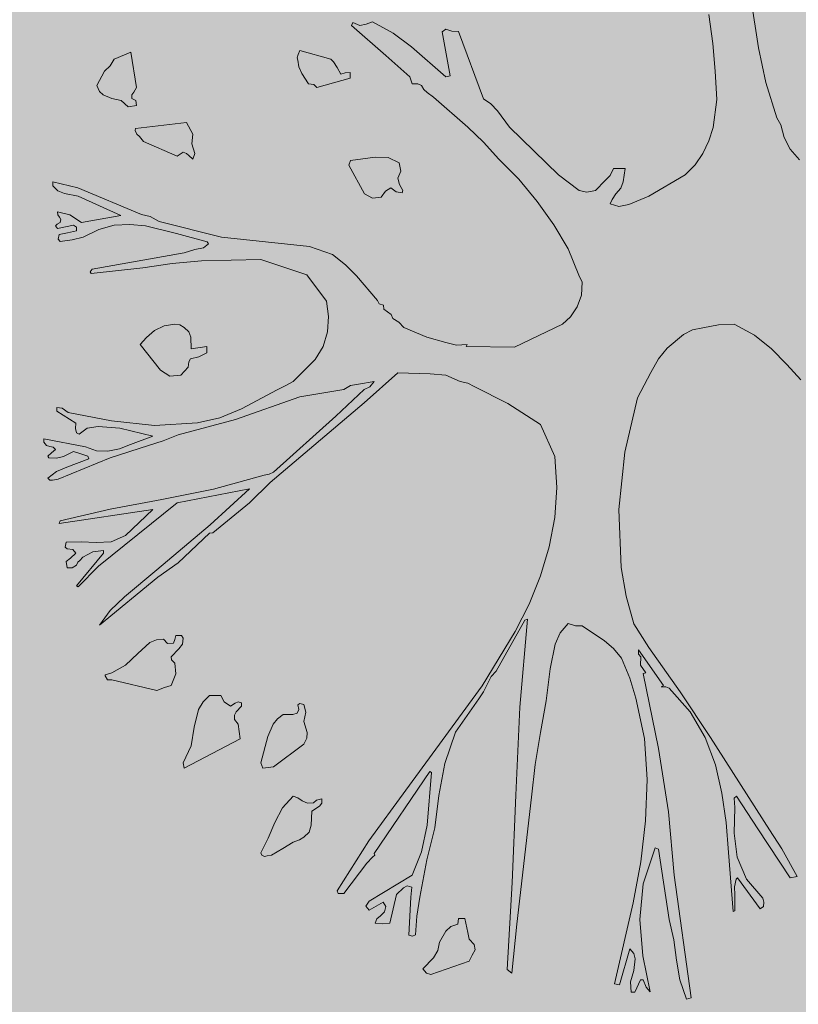
# Model space of a CAD drawing. Units: inches. Extents: x 84 to 1044, y -280 to 906.
# Tile 83 of 105: x 831.19 to 844.48, y 408.65 to 425.45. Entities that reach past the tile are written whole.
import ezdxf

# ---------------------------------------------------------------- set-up
doc = ezdxf.new("R2010")
doc.units = ezdxf.units.IN
doc.layers.add('A-ANNO-DIMS', color=2, linetype='Continuous', lineweight=18)
doc.layers.add('L-PLNT', color=114, linetype='Continuous', lineweight=15)
doc.layers.add('L-PLNT-PATT', color=9, linetype='Continuous', lineweight=9, true_color=0xafd9aa)
doc.styles.get("Standard").update_dxf_attribs({"font": 'arial.ttf'})
doc.dimstyles.get("Standard").update_dxf_attribs({"dimtxt": 0.18, "dimasz": 0.18, "dimexe": 0.18, "dimexo": 0.0625, "dimgap": 0.09, "dimtad": 0, "dimtih": 1, "dimtoh": 1, "dimdec": 4, "dimzin": 0, "dimdsep": 46, "dimtxsty": 'Standard', "dimcen": 0.09, "dimadec": 0, "dimazin": 0, "dimtfac": 1, "dimtdec": 4, "dimtofl": 0, "dimtmove": 0, "dimatfit": 3, "dimfxl": 1, "dimtolj": 1, "dimtzin": 0, "dimarcsym": 0})

# ---------------------------------------------------------------- blocks, each defined once
blk = doc.blocks.new('A$C37E508DF')
for p, q in [((0.7911, 1.1436), (0.8027, 1.0677)), ((0.7512, 1.0728), (0.7469, 1.1054)), ((0.3456, 1.093), (0.3469, 1.0964)), ((0.3469, 1.0964), (0.355, 1.093)), ((0.355, 1.093), (0.3619, 1.0943)), ((0.3619, 1.0943), (0.3692, 1.0968)), ((0.3692, 1.0968), (0.3923, 1.0844)), ((0.3842, 1.0591), (0.3456, 1.093)), ((0.3923, 1.0844), (0.4129, 1.069)), ((0.4472, 1.0857), (0.4515, 1.0887)), ((0.4562, 1.0364), (0.4472, 1.0857)), ((0.4515, 1.0887), (0.4584, 1.0865)), ((0.4584, 1.0865), (0.4657, 1.0861)), ((0.4657, 1.0861), (0.4939, 1.0107)), ((0.7538, 1.0415), (0.7512, 1.0728)), ((0.0789, 1.0552), (0.0978, 1.063)), ((0.0978, 1.063), (0.1042, 1.0231)), ((0.2856, 1.0604), (0.2877, 1.0647)), ((0.2877, 1.0647), (0.3224, 1.0552)), ((0.4129, 1.069), (0.4515, 1.0351)), ((0.8027, 1.0677), (0.8108, 1.0287)), ((0.0746, 1.0475), (0.0789, 1.0552)), ((0.2847, 1.0565), (0.2856, 1.0604)), ((0.2851, 1.054), (0.2847, 1.0565)), ((0.2864, 1.0463), (0.2851, 1.054)), ((0.3224, 1.0552), (0.3255, 1.0522)), ((0.3255, 1.0522), (0.3293, 1.0458)), ((0.4112, 1.0351), (0.3842, 1.0591)), ((0.0596, 1.0257), (0.0682, 1.0415)), ((0.0682, 1.0415), (0.0746, 1.0475)), ((0.2899, 1.039), (0.2864, 1.0463)), ((0.3293, 1.0458), (0.3336, 1.0381)), ((0.3336, 1.0381), (0.3383, 1.0398)), ((0.3383, 1.0398), (0.3439, 1.0402)), ((0.3439, 1.0402), (0.3439, 1.0338)), ((0.7559, 1.0098), (0.7538, 1.0415)), ((0.2972, 1.0274), (0.2899, 1.039)), ((0.3439, 1.0338), (0.3066, 1.0231)), ((0.4138, 1.0274), (0.4112, 1.0351)), ((0.4515, 1.0351), (0.4562, 1.0364)), ((0.8108, 1.0287), (0.8233, 0.9892)), ((0.0626, 1.0188), (0.0596, 1.0257)), ((0.0665, 1.0149), (0.0626, 1.0188)), ((0.1012, 1.018), (0.099, 1.0149)), ((0.1042, 1.0231), (0.1012, 1.018)), ((0.3032, 1.0265), (0.2972, 1.0274)), ((0.3066, 1.0231), (0.3032, 1.0265)), ((0.4202, 1.0274), (0.4138, 1.0274)), ((0.4241, 1.0257), (0.4202, 1.0274)), ((0.4267, 1.0209), (0.4241, 1.0257)), ((0.4305, 1.0175), (0.4267, 1.0209)), ((0.4378, 1.0124), (0.4305, 1.0175)), ((0.0763, 1.0111), (0.0665, 1.0149)), ((0.087, 1.0085), (0.0763, 1.0111)), ((0.0948, 1.0016), (0.087, 1.0085)), ((0.099, 1.0149), (0.099, 1.0111)), ((0.099, 1.0111), (0.1033, 1.0085)), ((0.1033, 1.0085), (0.1042, 1.0029)), ((0.476, 0.9789), (0.4378, 1.0124)), ((0.4939, 1.0107), (0.5021, 1.0051)), ((0.7516, 0.9785), (0.7559, 1.0098)), ((0.1042, 1.0029), (0.0948, 1.0016)), ((0.5021, 1.0051), (0.5094, 0.9969)), ((0.5094, 0.9969), (0.5231, 0.9789)), ((0.1029, 0.9772), (0.1604, 0.9841)), ((0.1604, 0.9841), (0.1672, 0.9708)), ((0.8233, 0.9892), (0.8275, 0.9815)), ((0.1025, 0.9751), (0.1029, 0.9772)), ((0.1046, 0.9708), (0.1025, 0.9751)), ((0.4939, 0.9618), (0.476, 0.9789)), ((0.5231, 0.9789), (0.578, 0.9253)), ((0.7469, 0.9635), (0.7516, 0.9785)), ((0.8275, 0.9815), (0.8314, 0.9673)), ((0.1076, 0.9682), (0.1046, 0.9708)), ((0.1119, 0.9626), (0.1076, 0.9682)), ((0.1496, 0.9463), (0.1119, 0.9626)), ((0.1672, 0.9708), (0.1664, 0.9601)), ((0.5111, 0.9429), (0.4939, 0.9618)), ((0.7401, 0.9493), (0.7469, 0.9635)), ((0.8314, 0.9673), (0.8383, 0.954)), ((0.1565, 0.9506), (0.1496, 0.9463)), ((0.1604, 0.9493), (0.1565, 0.9506)), ((0.1664, 0.9601), (0.1698, 0.9493)), ((0.8383, 0.954), (0.8486, 0.942)), ((0.1629, 0.9468), (0.1604, 0.9493)), ((0.1672, 0.9429), (0.1629, 0.9468)), ((0.1698, 0.9493), (0.1672, 0.9429)), ((0.3426, 0.936), (0.3443, 0.9412)), ((0.3443, 0.9412), (0.3722, 0.9451)), ((0.3722, 0.9451), (0.3868, 0.9446)), ((0.3868, 0.9446), (0.3992, 0.9386)), ((0.5334, 0.9202), (0.5111, 0.9429)), ((0.7315, 0.9365), (0.7401, 0.9493)), ((0.3602, 0.9039), (0.3426, 0.936)), ((0.4009, 0.9292), (0.3975, 0.9215)), ((0.3992, 0.9386), (0.4009, 0.9292)), ((0.6359, 0.9245), (0.6397, 0.9322)), ((0.6397, 0.9322), (0.653, 0.9322)), ((0.653, 0.9322), (0.6505, 0.9172)), ((0.7203, 0.9253), (0.7315, 0.9365)), ((0.3975, 0.9215), (0.3996, 0.9142)), ((0.554, 0.8953), (0.5334, 0.9202)), ((0.578, 0.9253), (0.6011, 0.9077)), ((0.6196, 0.9077), (0.6303, 0.9189)), ((0.6303, 0.9189), (0.6359, 0.9245)), ((0.6796, 0.9013), (0.7203, 0.9253)), ((0.0103, 0.9129), (0.0103, 0.9172)), ((0.0103, 0.9172), (0.0382, 0.9107)), ((0.0159, 0.9073), (0.0103, 0.9129)), ((0.0232, 0.9043), (0.0159, 0.9073)), ((0.0382, 0.9107), (0.1098, 0.8807)), ((0.3838, 0.9069), (0.379, 0.9)), ((0.3898, 0.9107), (0.3838, 0.9069)), ((0.3958, 0.906), (0.3898, 0.9107)), ((0.3996, 0.9142), (0.4031, 0.9077)), ((0.4031, 0.9077), (0.4026, 0.9052)), ((0.6011, 0.9077), (0.6097, 0.9056)), ((0.6097, 0.9056), (0.6196, 0.9077)), ((0.6479, 0.9103), (0.6423, 0.9039)), ((0.6505, 0.9172), (0.6479, 0.9103)), ((0.0386, 0.9013), (0.0232, 0.9043)), ((0.0866, 0.8794), (0.0386, 0.9013)), ((0.3692, 0.8992), (0.3602, 0.9039)), ((0.379, 0.9), (0.3692, 0.8992)), ((0.4026, 0.9052), (0.3958, 0.906)), ((0.5728, 0.8691), (0.554, 0.8953)), ((0.6384, 0.8974), (0.6359, 0.8927)), ((0.6423, 0.9039), (0.6384, 0.8974)), ((0.6569, 0.8919), (0.6796, 0.9013)), ((0.6359, 0.8927), (0.6457, 0.8897)), ((0.6457, 0.8897), (0.6569, 0.8919)), ((0.0159, 0.8803), (0.0154, 0.8837)), ((0.0154, 0.8837), (0.0292, 0.8803)), ((0.0176, 0.8777), (0.0159, 0.8803)), ((0.0193, 0.8752), (0.0176, 0.8777)), ((0.0184, 0.8717), (0.0193, 0.8752)), ((0.0292, 0.8803), (0.0424, 0.8717)), ((0.0424, 0.8717), (0.0866, 0.8794)), ((0.1098, 0.8807), (0.1196, 0.8786)), ((0.1196, 0.8786), (0.1295, 0.873)), ((0.0133, 0.8679), (0.015, 0.87)), ((0.0154, 0.8649), (0.0133, 0.8679)), ((0.015, 0.87), (0.0184, 0.8717)), ((0.0334, 0.8687), (0.0154, 0.8649)), ((0.0266, 0.8602), (0.0369, 0.8623)), ((0.0369, 0.8666), (0.0334, 0.8687)), ((0.0369, 0.8623), (0.0369, 0.8666)), ((0.0617, 0.864), (0.0442, 0.8554)), ((0.0789, 0.8687), (0.0617, 0.864)), ((0.0965, 0.8696), (0.0789, 0.8687)), ((0.1141, 0.8679), (0.0965, 0.8696)), ((0.1492, 0.8593), (0.1141, 0.8679)), ((0.1295, 0.873), (0.1994, 0.8554)), ((0.5887, 0.8421), (0.5728, 0.8691)), ((0.0163, 0.8529), (0.0171, 0.8584)), ((0.0184, 0.8503), (0.0163, 0.8529)), ((0.0171, 0.8584), (0.0266, 0.8602)), ((0.0317, 0.8524), (0.0184, 0.8503)), ((0.0442, 0.8554), (0.0317, 0.8524)), ((0.1835, 0.8499), (0.1492, 0.8593)), ((0.1994, 0.8554), (0.2984, 0.8447)), ((0.1578, 0.8378), (0.1698, 0.8413)), ((0.1698, 0.8413), (0.1792, 0.8434)), ((0.1792, 0.8434), (0.1848, 0.8477)), ((0.1848, 0.8477), (0.1835, 0.8499)), ((0.2984, 0.8447), (0.3242, 0.8357)), ((0.6007, 0.8125), (0.5887, 0.8421)), ((0.0545, 0.8194), (0.1578, 0.8378)), ((0.2436, 0.8301), (0.1771, 0.8288)), ((0.2954, 0.813), (0.2436, 0.8301)), ((0.3242, 0.8357), (0.3387, 0.8241)), ((0.0519, 0.8164), (0.0545, 0.8194)), ((0.1111, 0.8207), (0.0532, 0.8143)), ((0.1441, 0.8258), (0.1111, 0.8207)), ((0.1771, 0.8288), (0.1441, 0.8258)), ((0.3387, 0.8241), (0.3512, 0.8117)), ((0.0532, 0.8143), (0.0519, 0.8164)), ((0.3173, 0.7834), (0.2954, 0.813)), ((0.3512, 0.8117), (0.3748, 0.7842)), ((0.6046, 0.8048), (0.6007, 0.8125)), ((0.6037, 0.7903), (0.6046, 0.8048)), ((0.599, 0.777), (0.6037, 0.7903)), ((0.3199, 0.7662), (0.3173, 0.7834)), ((0.3748, 0.7842), (0.3765, 0.7804)), ((0.3765, 0.7804), (0.3816, 0.7791)), ((0.3816, 0.7791), (0.382, 0.7744)), ((0.382, 0.7744), (0.3859, 0.7714)), ((0.5913, 0.7658), (0.599, 0.777)), ((0.3186, 0.7491), (0.3199, 0.7662)), ((0.3859, 0.7714), (0.3902, 0.7684)), ((0.3902, 0.7684), (0.3919, 0.7641)), ((0.3919, 0.7641), (0.3988, 0.7598)), ((0.5823, 0.7577), (0.5913, 0.7658)), ((0.1244, 0.7504), (0.1351, 0.7559)), ((0.1351, 0.7559), (0.1471, 0.7577)), ((0.1471, 0.7577), (0.1527, 0.7568)), ((0.1527, 0.7568), (0.1578, 0.7538)), ((0.1578, 0.7538), (0.1629, 0.7491)), ((0.3988, 0.7598), (0.4043, 0.7538)), ((0.4043, 0.7538), (0.4301, 0.7431)), ((0.5287, 0.7319), (0.5823, 0.7577)), ((0.7401, 0.7534), (0.7285, 0.7512)), ((0.7577, 0.7568), (0.7401, 0.7534)), ((0.7752, 0.7577), (0.7577, 0.7568)), ((0.798, 0.7452), (0.7752, 0.7577)), ((0.1081, 0.7349), (0.1153, 0.7427)), ((0.1153, 0.7427), (0.1244, 0.7504)), ((0.1629, 0.7491), (0.1651, 0.7431)), ((0.1651, 0.7431), (0.1655, 0.7298)), ((0.3139, 0.7324), (0.3186, 0.7491)), ((0.4301, 0.7431), (0.4515, 0.7371)), ((0.7182, 0.7461), (0.7002, 0.7307)), ((0.7285, 0.7512), (0.7182, 0.7461)), ((0.8173, 0.7298), (0.798, 0.7452)), ((0.1312, 0.7058), (0.1081, 0.7349)), ((0.1655, 0.7298), (0.1831, 0.7324)), ((0.1831, 0.7324), (0.1831, 0.7255)), ((0.3049, 0.7178), (0.3139, 0.7324)), ((0.4515, 0.7371), (0.4635, 0.7341)), ((0.4635, 0.7341), (0.4755, 0.7349)), ((0.4755, 0.7349), (0.4742, 0.7324)), ((0.4742, 0.7324), (0.5287, 0.7319)), ((0.7002, 0.7307), (0.6903, 0.7186)), ((0.8344, 0.7122), (0.8173, 0.7298)), ((0.1646, 0.7186), (0.1629, 0.7152)), ((0.1741, 0.7208), (0.1646, 0.7186)), ((0.1831, 0.7255), (0.1741, 0.7208)), ((0.6903, 0.7186), (0.6818, 0.7032)), ((0.1621, 0.7092), (0.1539, 0.7002)), ((0.1629, 0.7152), (0.1621, 0.7092)), ((0.28, 0.6933), (0.3049, 0.7178)), ((0.8503, 0.6951), (0.8344, 0.7122)), ((0.1415, 0.6994), (0.1312, 0.7058)), ((0.1539, 0.7002), (0.1415, 0.6994)), ((0.3975, 0.7028), (0.3598, 0.6693)), ((0.4339, 0.7019), (0.3975, 0.7028)), ((0.4515, 0.7002), (0.4339, 0.7019)), ((0.4674, 0.6933), (0.4515, 0.7002)), ((0.6818, 0.7032), (0.6667, 0.6749)), ((0.262, 0.6839), (0.271, 0.6882)), ((0.271, 0.6882), (0.28, 0.6933)), ((0.3443, 0.6886), (0.337, 0.6843)), ((0.3533, 0.6903), (0.3443, 0.6886)), ((0.3709, 0.6933), (0.3533, 0.6903)), ((0.3598, 0.6843), (0.3662, 0.6873)), ((0.3662, 0.6873), (0.3709, 0.6933)), ((0.476, 0.6912), (0.4674, 0.6933)), ((0.4832, 0.6878), (0.476, 0.6912)), ((0.521, 0.6685), (0.4832, 0.6878)), ((0.2877, 0.6762), (0.2152, 0.6505)), ((0.2221, 0.6625), (0.262, 0.6839)), ((0.337, 0.6843), (0.2877, 0.6762)), ((0.328, 0.6543), (0.3598, 0.6843)), ((0.6667, 0.6749), (0.6526, 0.614)), ((0.0146, 0.6599), (0.0146, 0.6642)), ((0.0146, 0.6642), (0.0206, 0.6633)), ((0.0206, 0.6633), (0.0274, 0.6586)), ((0.3598, 0.6693), (0.2543, 0.5797)), ((0.5578, 0.6449), (0.521, 0.6685)), ((0.036, 0.6466), (0.0146, 0.6599)), ((0.0274, 0.6586), (0.0759, 0.6492)), ((0.1728, 0.647), (0.1977, 0.6526)), ((0.1977, 0.6526), (0.2221, 0.6625)), ((0.2581, 0.5913), (0.328, 0.6543)), ((0.0356, 0.6406), (0.036, 0.6466)), ((0.0609, 0.6428), (0.0489, 0.641)), ((0.0853, 0.641), (0.0609, 0.6428)), ((0.0759, 0.6492), (0.1244, 0.644)), ((0.1244, 0.644), (0.1728, 0.647)), ((0.2152, 0.6505), (0.1509, 0.6333)), ((0.5737, 0.6089), (0.5578, 0.6449)), ((0.0369, 0.6355), (0.0356, 0.6406)), ((0.0399, 0.6342), (0.0369, 0.6355)), ((0.0489, 0.641), (0.0399, 0.6342)), ((0.1226, 0.632), (0.0853, 0.641)), ((0.0973, 0.6226), (0.1226, 0.632)), ((0.1509, 0.6333), (0.1342, 0.6265)), ((0, 0.629), (0.0467, 0.62)), ((0, 0.6252), (0, 0.629)), ((0.003, 0.6213), (0, 0.6252)), ((0.0069, 0.6204), (0.003, 0.6213)), ((0.0107, 0.6196), (0.0069, 0.6204)), ((0.0133, 0.617), (0.0107, 0.6196)), ((0.0467, 0.62), (0.0592, 0.6153)), ((0.1175, 0.6213), (0.0746, 0.6076)), ((0.0849, 0.6175), (0.0973, 0.6226)), ((0.1342, 0.6265), (0.1175, 0.6213)), ((0.0047, 0.6093), (0.0086, 0.6132)), ((0.0056, 0.6076), (0.0047, 0.6093)), ((0.0086, 0.6132), (0.0133, 0.617)), ((0.0223, 0.6089), (0.0141, 0.6072)), ((0.0334, 0.6145), (0.0223, 0.6089)), ((0.0416, 0.6119), (0.0334, 0.6145)), ((0.0493, 0.6093), (0.0416, 0.6119)), ((0.0506, 0.6063), (0.0493, 0.6093)), ((0.0592, 0.6153), (0.072, 0.6149)), ((0.072, 0.6149), (0.0849, 0.6175)), ((0.5763, 0.5741), (0.5737, 0.6089)), ((0.6526, 0.614), (0.6457, 0.5497)), ((0.0141, 0.6072), (0.0056, 0.6076)), ((0.0141, 0.5921), (0.0257, 0.5969)), ((0.0746, 0.6076), (0.0163, 0.5836)), ((0.0257, 0.5969), (0.0506, 0.6063)), ((0.0047, 0.5849), (0.0141, 0.5921)), ((0.1904, 0.5724), (0.2474, 0.5879)), ((0.2474, 0.5879), (0.253, 0.5892)), ((0.253, 0.5892), (0.2581, 0.5913)), ((0.0069, 0.5823), (0.0047, 0.5849)), ((0.0099, 0.5823), (0.0069, 0.5823)), ((0.0163, 0.5836), (0.0099, 0.5823)), ((0.2543, 0.5797), (0.2311, 0.557)), ((0.1325, 0.5608), (0.1904, 0.5724)), ((0.2311, 0.5729), (0.1496, 0.557)), ((0.1869, 0.5325), (0.2311, 0.5729)), ((0.5737, 0.5407), (0.5763, 0.5741)), ((0.1496, 0.557), (0.0613, 0.4858)), ((0.0746, 0.5501), (0.1325, 0.5608)), ((0.2311, 0.557), (0.1899, 0.5235)), ((0.1226, 0.5497), (0.0171, 0.5338)), ((0.0184, 0.5368), (0.0746, 0.5501)), ((0.0917, 0.5205), (0.1226, 0.5497)), ((0.6457, 0.5497), (0.6483, 0.4845)), ((0.0171, 0.5338), (0.0184, 0.5368)), ((0.1269, 0.482), (0.1869, 0.5325)), ((0.5677, 0.5077), (0.5737, 0.5407)), ((0.0755, 0.5133), (0.0917, 0.5205)), ((0.1861, 0.5231), (0.1509, 0.4897)), ((0.1899, 0.5235), (0.1861, 0.5231)), ((0.024, 0.5072), (0.0253, 0.5128)), ((0.0253, 0.5128), (0.042, 0.5133)), ((0.042, 0.5133), (0.0587, 0.5124)), ((0.0587, 0.5124), (0.0755, 0.5133)), ((0.0262, 0.5055), (0.024, 0.5072)), ((0.0326, 0.5047), (0.0262, 0.5055)), ((0.03, 0.4948), (0.036, 0.5004)), ((0.036, 0.5004), (0.0326, 0.5047)), ((0.0369, 0.4639), (0.0669, 0.5004)), ((0.0549, 0.5021), (0.0437, 0.4961)), ((0.0669, 0.5034), (0.0549, 0.5021)), ((0.0669, 0.5004), (0.0669, 0.5034)), ((0.5578, 0.4751), (0.5677, 0.5077)), ((0.0253, 0.491), (0.03, 0.4948)), ((0.0262, 0.4841), (0.0253, 0.491)), ((0.0369, 0.4871), (0.0317, 0.4841)), ((0.0382, 0.4905), (0.0369, 0.4871)), ((0.0403, 0.4922), (0.0382, 0.4905)), ((0.0437, 0.4961), (0.0403, 0.4922)), ((0.1509, 0.4897), (0.1282, 0.4734)), ((0.0317, 0.4841), (0.0262, 0.4841)), ((0.0613, 0.4858), (0.0386, 0.4627)), ((0.0905, 0.4515), (0.1269, 0.482)), ((0.6483, 0.4845), (0.6539, 0.4524)), ((0.1282, 0.4734), (0.0626, 0.4198)), ((0.545, 0.4434), (0.5578, 0.4751)), ((0.0386, 0.4627), (0.0369, 0.4639)), ((0.0746, 0.4361), (0.0905, 0.4515)), ((0.5295, 0.4125), (0.545, 0.4434)), ((0.6539, 0.4524), (0.6625, 0.4211)), ((0.0626, 0.4198), (0.0746, 0.4361)), ((0.5403, 0.4254), (0.5081, 0.3679)), ((0.5347, 0.3276), (0.5433, 0.4266)), ((0.5433, 0.4266), (0.5403, 0.4254)), ((0.5887, 0.4215), (0.5797, 0.4112)), ((0.5969, 0.4189), (0.5887, 0.4215)), ((0.6625, 0.4211), (0.6796, 0.3945)), ((0.4922, 0.3516), (0.5295, 0.4125)), ((0.5797, 0.4112), (0.5741, 0.3983)), ((0.6046, 0.4189), (0.5969, 0.4189)), ((0.6295, 0.4022), (0.6046, 0.4189)), ((0.1055, 0.388), (0.1192, 0.4001)), ((0.1192, 0.4001), (0.1265, 0.4031)), ((0.1265, 0.4031), (0.1346, 0.4039)), ((0.1346, 0.4039), (0.1389, 0.3992)), ((0.1389, 0.3992), (0.1458, 0.3996)), ((0.1458, 0.3996), (0.1471, 0.4035)), ((0.1471, 0.4035), (0.1484, 0.4082)), ((0.1484, 0.4082), (0.1548, 0.4082)), ((0.1556, 0.3983), (0.1518, 0.3932)), ((0.1548, 0.4082), (0.1565, 0.4052)), ((0.1565, 0.4052), (0.1556, 0.3983)), ((0.5741, 0.3983), (0.5686, 0.3705)), ((0.6397, 0.3936), (0.6295, 0.4022)), ((0.0917, 0.3748), (0.1055, 0.388)), ((0.1518, 0.3932), (0.1432, 0.3842)), ((0.6487, 0.3825), (0.6397, 0.3936)), ((0.6959, 0.352), (0.668, 0.3919)), ((0.668, 0.3919), (0.668, 0.3872)), ((0.668, 0.3872), (0.6706, 0.3842)), ((0.6796, 0.3945), (0.7148, 0.3447)), ((0.1432, 0.3842), (0.1436, 0.3808)), ((0.1436, 0.3808), (0.1471, 0.3769)), ((0.1471, 0.3769), (0.1484, 0.3649)), ((0.6582, 0.3602), (0.6487, 0.3825)), ((0.6706, 0.3842), (0.6702, 0.3748)), ((0.069, 0.364), (0.0763, 0.3662)), ((0.0763, 0.3662), (0.0917, 0.3748)), ((0.1484, 0.3649), (0.1432, 0.352)), ((0.5081, 0.3679), (0.5025, 0.3619)), ((0.5686, 0.3705), (0.5643, 0.3349)), ((0.6702, 0.3748), (0.6762, 0.3662)), ((0.6762, 0.3662), (0.6732, 0.3653)), ((0.6732, 0.3653), (0.6903, 0.2813)), ((0.069, 0.3627), (0.069, 0.364)), ((0.0716, 0.3585), (0.069, 0.3627)), ((0.0763, 0.3585), (0.0716, 0.3585)), ((0.1269, 0.3464), (0.0763, 0.3585)), ((0.4982, 0.3537), (0.4939, 0.3447)), ((0.5025, 0.3619), (0.4982, 0.3537)), ((0.665, 0.3379), (0.6582, 0.3602)), ((0.1355, 0.3499), (0.1269, 0.3464)), ((0.1432, 0.352), (0.1355, 0.3499)), ((0.4065, 0.2345), (0.4922, 0.3516)), ((0.4939, 0.3447), (0.4884, 0.337)), ((0.6933, 0.3503), (0.6959, 0.352)), ((0.6985, 0.3503), (0.6933, 0.3503)), ((0.7023, 0.349), (0.6985, 0.3503)), ((0.7259, 0.3224), (0.7023, 0.349)), ((0.7148, 0.3447), (0.7487, 0.2937)), ((0.1737, 0.325), (0.1788, 0.3336)), ((0.1788, 0.3336), (0.1861, 0.3409)), ((0.1861, 0.3409), (0.199, 0.3409)), ((0.199, 0.3409), (0.2024, 0.3336)), ((0.2024, 0.3336), (0.2097, 0.3289)), ((0.2097, 0.3289), (0.2148, 0.3323)), ((0.2148, 0.3323), (0.2182, 0.3336)), ((0.2182, 0.3336), (0.2221, 0.3327)), ((0.2221, 0.3327), (0.2221, 0.3289)), ((0.2851, 0.3302), (0.2877, 0.3319)), ((0.2877, 0.3319), (0.292, 0.3306)), ((0.4884, 0.337), (0.4622, 0.2997)), ((0.5643, 0.3349), (0.5578, 0.2993)), ((0.6745, 0.2924), (0.665, 0.3379)), ((0.1689, 0.3053), (0.1737, 0.325)), ((0.2161, 0.3224), (0.214, 0.3186)), ((0.2221, 0.3289), (0.2161, 0.3224)), ((0.2796, 0.3194), (0.2847, 0.3211)), ((0.2847, 0.3211), (0.2864, 0.325)), ((0.2864, 0.325), (0.2851, 0.3302)), ((0.292, 0.3306), (0.2941, 0.322)), ((0.2941, 0.322), (0.292, 0.3117)), ((0.53, 0.229), (0.5347, 0.3276)), ((0.7427, 0.2937), (0.7259, 0.3224)), ((0.214, 0.3186), (0.214, 0.3139)), ((0.214, 0.3139), (0.2182, 0.3087)), ((0.2577, 0.3087), (0.2624, 0.3147)), ((0.2624, 0.3147), (0.2689, 0.3194)), ((0.2689, 0.3194), (0.2796, 0.3194)), ((0.292, 0.3117), (0.2959, 0.2993)), ((0.1655, 0.2843), (0.1689, 0.3053)), ((0.2182, 0.3087), (0.2204, 0.292)), ((0.2517, 0.2946), (0.2577, 0.3087)), ((0.2959, 0.2993), (0.2954, 0.2928)), ((0.4622, 0.2997), (0.4502, 0.2645)), ((0.5578, 0.2993), (0.5518, 0.2633)), ((0.2204, 0.292), (0.1578, 0.259)), ((0.2436, 0.265), (0.2517, 0.2946)), ((0.2954, 0.2928), (0.292, 0.286)), ((0.6775, 0.2465), (0.6745, 0.2924)), ((0.7542, 0.2628), (0.7427, 0.2937)), ((0.7487, 0.2937), (0.8151, 0.1899)), ((0.1565, 0.265), (0.1655, 0.2843)), ((0.292, 0.286), (0.2581, 0.2607)), ((0.6903, 0.2813), (0.7015, 0.2101)), ((0.1578, 0.259), (0.1565, 0.265)), ((0.2461, 0.259), (0.2436, 0.265)), ((0.2581, 0.2607), (0.2461, 0.259)), ((0.4335, 0.2556), (0.3709, 0.1634)), ((0.4305, 0.1951), (0.4352, 0.2543)), ((0.4352, 0.2543), (0.4335, 0.2556)), ((0.4502, 0.2645), (0.4438, 0.2285)), ((0.5518, 0.2633), (0.5475, 0.2268)), ((0.7615, 0.2311), (0.7542, 0.2628)), ((0.6758, 0.2002), (0.6775, 0.2465)), ((0.3649, 0.1775), (0.4065, 0.2345)), ((0.268, 0.2148), (0.28, 0.2277)), ((0.28, 0.2277), (0.2851, 0.226)), ((0.2851, 0.226), (0.2903, 0.2225)), ((0.2903, 0.2225), (0.2963, 0.22)), ((0.3027, 0.2204), (0.3061, 0.2234)), ((0.3061, 0.2234), (0.3122, 0.2247)), ((0.3122, 0.2247), (0.3122, 0.22)), ((0.4438, 0.2285), (0.4391, 0.1921)), ((0.5261, 0.1308), (0.53, 0.229)), ((0.5475, 0.2268), (0.5313, 0.084)), ((0.7662, 0.1981), (0.7615, 0.2311)), ((0.7778, 0.2277), (0.7752, 0.2255)), ((0.7752, 0.2255), (0.7761, 0.2152)), ((0.8018, 0.1912), (0.7778, 0.2277)), ((0.2594, 0.1981), (0.268, 0.2148)), ((0.2963, 0.22), (0.3027, 0.2204)), ((0.301, 0.211), (0.3002, 0.1951)), ((0.3096, 0.2165), (0.301, 0.211)), ((0.3122, 0.22), (0.3096, 0.2165)), ((0.7015, 0.2101), (0.7079, 0.1389)), ((0.7761, 0.2152), (0.7752, 0.1861)), ((0.6706, 0.1539), (0.6758, 0.2002)), ((0.2521, 0.1805), (0.2594, 0.1981)), ((0.3002, 0.1951), (0.298, 0.1874)), ((0.4241, 0.1651), (0.4305, 0.1951)), ((0.4391, 0.1921), (0.4301, 0.1561)), ((0.7688, 0.1646), (0.7662, 0.1981)), ((0.8383, 0.1359), (0.8018, 0.1912)), ((0.8151, 0.1899), (0.8288, 0.1685)), ((0.2436, 0.1642), (0.2521, 0.1805)), ((0.2873, 0.1788), (0.28, 0.1762)), ((0.292, 0.1818), (0.2873, 0.1788)), ((0.298, 0.1874), (0.292, 0.1818)), ((0.3293, 0.1213), (0.3649, 0.1775)), ((0.7752, 0.1861), (0.7787, 0.1591)), ((0.2684, 0.1689), (0.2556, 0.1616)), ((0.28, 0.1762), (0.2684, 0.1689)), ((0.6865, 0.1698), (0.6732, 0.1295)), ((0.6903, 0.1681), (0.6865, 0.1698)), ((0.7023, 0.0892), (0.6903, 0.1681)), ((0.8288, 0.1685), (0.846, 0.1376)), ((0.2448, 0.1616), (0.2436, 0.1642)), ((0.2478, 0.1599), (0.2448, 0.1616)), ((0.2508, 0.1608), (0.2478, 0.1599)), ((0.2556, 0.1616), (0.2508, 0.1608)), ((0.3692, 0.1591), (0.3628, 0.1526)), ((0.3718, 0.1616), (0.3692, 0.1591)), ((0.3709, 0.1634), (0.3718, 0.1616)), ((0.4138, 0.1389), (0.4241, 0.1651)), ((0.4301, 0.1561), (0.4224, 0.1145)), ((0.774, 0.0982), (0.7688, 0.1646)), ((0.7787, 0.1591), (0.789, 0.1346)), ((0.3628, 0.1526), (0.337, 0.1183)), ((0.662, 0.108), (0.6706, 0.1539)), ((0.3653, 0.1098), (0.4138, 0.1389)), ((0.7079, 0.1389), (0.7268, 0.0013)), ((0.7774, 0.1346), (0.7757, 0.1261)), ((0.7791, 0.1359), (0.7774, 0.1346)), ((0.8044, 0.1012), (0.7791, 0.1359)), ((0.789, 0.1346), (0.8074, 0.1132)), ((0.846, 0.1376), (0.8383, 0.1359)), ((0.4039, 0.1248), (0.3962, 0.1175)), ((0.4082, 0.1269), (0.4039, 0.1248)), ((0.4134, 0.1256), (0.4082, 0.1269)), ((0.4121, 0.1145), (0.4134, 0.1256)), ((0.5205, 0.033), (0.5261, 0.1308)), ((0.6732, 0.1295), (0.6693, 0.0892)), ((0.7757, 0.1261), (0.7761, 0.117)), ((0.3306, 0.1183), (0.3293, 0.1213)), ((0.337, 0.1183), (0.3306, 0.1183)), ((0.3962, 0.1175), (0.3885, 0.0853)), ((0.4099, 0.0716), (0.4121, 0.1145)), ((0.4224, 0.1145), (0.4189, 0.093)), ((0.7761, 0.117), (0.7761, 0.099)), ((0.8074, 0.1132), (0.8087, 0.1089)), ((0.3615, 0.1042), (0.3653, 0.1098)), ((0.3653, 0.0999), (0.3615, 0.1042)), ((0.3812, 0.1089), (0.3653, 0.0999)), ((0.3842, 0.1037), (0.3812, 0.1089)), ((0.3825, 0.0978), (0.3842, 0.1037)), ((0.641, 0.0172), (0.662, 0.108)), ((0.8083, 0.1037), (0.8044, 0.1012)), ((0.8087, 0.1089), (0.8083, 0.1037)), ((0.3722, 0.0853), (0.3739, 0.09)), ((0.3739, 0.09), (0.3782, 0.0935)), ((0.3782, 0.0935), (0.3825, 0.0978)), ((0.4189, 0.093), (0.4176, 0.072)), ((0.4648, 0.084), (0.4657, 0.0905)), ((0.4657, 0.0905), (0.473, 0.0905)), ((0.473, 0.0905), (0.476, 0.0746)), ((0.6693, 0.0892), (0.6728, 0.0484)), ((0.7075, 0.0665), (0.7023, 0.0892)), ((0.7761, 0.099), (0.774, 0.0982)), ((0.3808, 0.0845), (0.3722, 0.0853)), ((0.3885, 0.0853), (0.3808, 0.0845)), ((0.4515, 0.0763), (0.4571, 0.0815)), ((0.4571, 0.0815), (0.4648, 0.084)), ((0.5313, 0.084), (0.5257, 0.0291)), ((0.4142, 0.0707), (0.4099, 0.0716)), ((0.4176, 0.072), (0.4142, 0.0707)), ((0.4442, 0.0639), (0.4515, 0.0763)), ((0.476, 0.0746), (0.4777, 0.0673)), ((0.4777, 0.0673), (0.4832, 0.0613)), ((0.7105, 0.0437), (0.7075, 0.0665)), ((0.4425, 0.0544), (0.4442, 0.0639)), ((0.4845, 0.0553), (0.4811, 0.0493)), ((0.4832, 0.0613), (0.4845, 0.0553)), ((0.6582, 0.0562), (0.6466, 0.0159)), ((0.6625, 0.051), (0.6582, 0.0562)), ((0.4258, 0.0339), (0.4378, 0.0463)), ((0.4378, 0.0463), (0.4425, 0.0544)), ((0.4811, 0.0493), (0.4777, 0.0424)), ((0.6642, 0.045), (0.6625, 0.051)), ((0.6625, 0.0321), (0.6642, 0.045)), ((0.6728, 0.0484), (0.6809, 0.0082)), ((0.4296, 0.0291), (0.4258, 0.0339)), ((0.4777, 0.0424), (0.4348, 0.0274)), ((0.7144, 0.0214), (0.7105, 0.0437)), ((0.4348, 0.0274), (0.4296, 0.0291)), ((0.5257, 0.0291), (0.5205, 0.033)), ((0.659, 0.0193), (0.6625, 0.0321)), ((0.6466, 0.0159), (0.641, 0.0172)), ((0.6595, 0.0077), (0.659, 0.0193)), ((0.6702, 0.0214), (0.6637, 0.0077)), ((0.6732, 0.0214), (0.6702, 0.0214)), ((0.6766, 0.0133), (0.6732, 0.0214)), ((0.6809, 0.0082), (0.6766, 0.0133)), ((0.7216, 0), (0.7144, 0.0214)), ((0.6637, 0.0077), (0.6595, 0.0077)), ((0.7268, 0.0013), (0.7216, 0))]:
    blk.add_line(p, q)
blk = doc.blocks.new('*D62')
at = {"layer": 'A-ANNO-DIMS', "color": 0, "lineweight": -2, "transparency": 16777216}
for p, q in [((203.179, 709.183), (203.179, 905.9)), ((896.074, 400.183), (896.074, 905.9)), ((203.359, 905.72), (549.232, 905.72)), ((895.894, 905.72), (550.021, 905.72))]:
    blk.add_line(p, q, dxfattribs=at)
at = {"layer": 'A-ANNO-DIMS', "color": 0, "transparency": 16777216}
for points in [[(203.359, 905.75), (203.359, 905.69), (203.179, 905.72)], [(895.894, 905.75), (895.894, 905.69), (896.074, 905.72)]]:
    blk.add_solid(points, dxfattribs=at)
at = {"layer": 'Defpoints', "color": 0, "transparency": 16777216}
for p in [(896.074, 905.72), (203.179, 709.12), (896.074, 400.12)]:
    blk.add_point(p, dxfattribs=at)
at = {"layer": 'A-ANNO-DIMS', "color": 0, "transparency": 16777216, "insert": (549.627, 905.72), "char_height": 0.18, "attachment_point": 5}
blk.add_mtext('\\A1;692.9', dxfattribs=at)
blk = doc.blocks.new('*D63')
at = {"layer": 'A-ANNO-DIMS', "color": 0, "lineweight": -2, "transparency": 16777216}
for p, q in [((833.136, 709.12), (1043.768, 709.12)), ((1043.588, 708.94), (1043.588, 400.302)), ((1043.588, 91.3), (1043.588, 399.938)), ((896.136, 91.12), (1043.768, 91.12))]:
    blk.add_line(p, q, dxfattribs=at)
at = {"layer": 'A-ANNO-DIMS', "color": 0, "transparency": 16777216}
for points in [[(1043.558, 708.94), (1043.618, 708.94), (1043.588, 709.12)], [(1043.558, 91.3), (1043.618, 91.3), (1043.588, 91.12)]]:
    blk.add_solid(points, dxfattribs=at)
at = {"layer": 'Defpoints', "color": 0, "transparency": 16777216}
for p in [(833.074, 709.12), (1043.588, 709.12), (896.074, 91.12)]:
    blk.add_point(p, dxfattribs=at)
at = {"layer": 'A-ANNO-DIMS', "color": 0, "transparency": 16777216, "insert": (1043.588, 400.12), "char_height": 0.18, "attachment_point": 5}
blk.add_mtext('\\A1;618', dxfattribs=at)

msp = doc.modelspace()

# ---------------------------------------------------------------- hatches: boundary and pattern name
at = {"layer": 'L-PLNT-PATT', "transparency": 33554597}
h = msp.add_hatch(color=256, dxfattribs=at)
h.dxf.hatch_style = 1
h.paths.add_polyline_path([(896.074, 511.12), (704.074, 511.12), (704.074, 491.62), (704.074, 419.62), (704.074, 400.12), (833.074, 400.12), (896.074, 400.12)])

# ---------------------------------------------------------------- block references
at = {"layer": 'L-PLNT', "xscale": 15.19586232982809, "yscale": 15.19586232982809, "zscale": 15.19586232982809}
msp.add_blockref('A$C37E508DF', (831.605, 408.742), dxfattribs=at)

# ---------------------------------------------------------------- dimensions: what is measured, and where the dimension line sits
at = {"layer": 'A-ANNO-DIMS'}
dim = msp.add_linear_dim(base=(896.074, 905.72), p1=(203.179, 709.12), p2=(896.074, 400.12), dimstyle='Standard', override={"dimdec": 1, "dimlfac": 1, "dimrnd": 0, "dimzin": 0, "dimdsep": 46, "dimlunit": 2}, dxfattribs=at)
dim.commit()
dim.dimension.update_dxf_attribs({"geometry": '*D62', "text_midpoint": (549.627, 905.72)})
dim = msp.add_linear_dim(base=(1043.588, 709.12), p1=(896.074, 91.12), p2=(833.074, 709.12), angle=90, dimstyle='Standard', override={"dimdec": 0, "dimlfac": 1, "dimrnd": 0, "dimzin": 0, "dimdsep": 46, "dimlunit": 2}, dxfattribs=at)
dim.commit()
dim.dimension.update_dxf_attribs({"geometry": '*D63', "text_midpoint": (1043.588, 400.12)})

doc.saveas('drawing.dxf')
